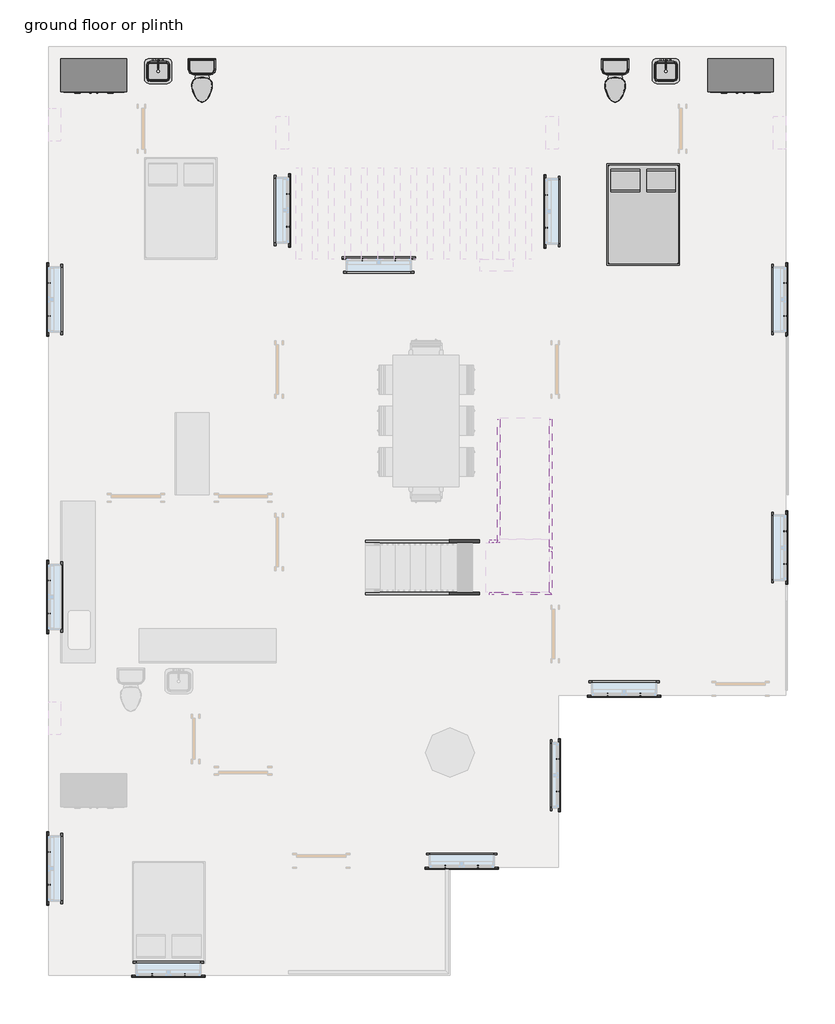
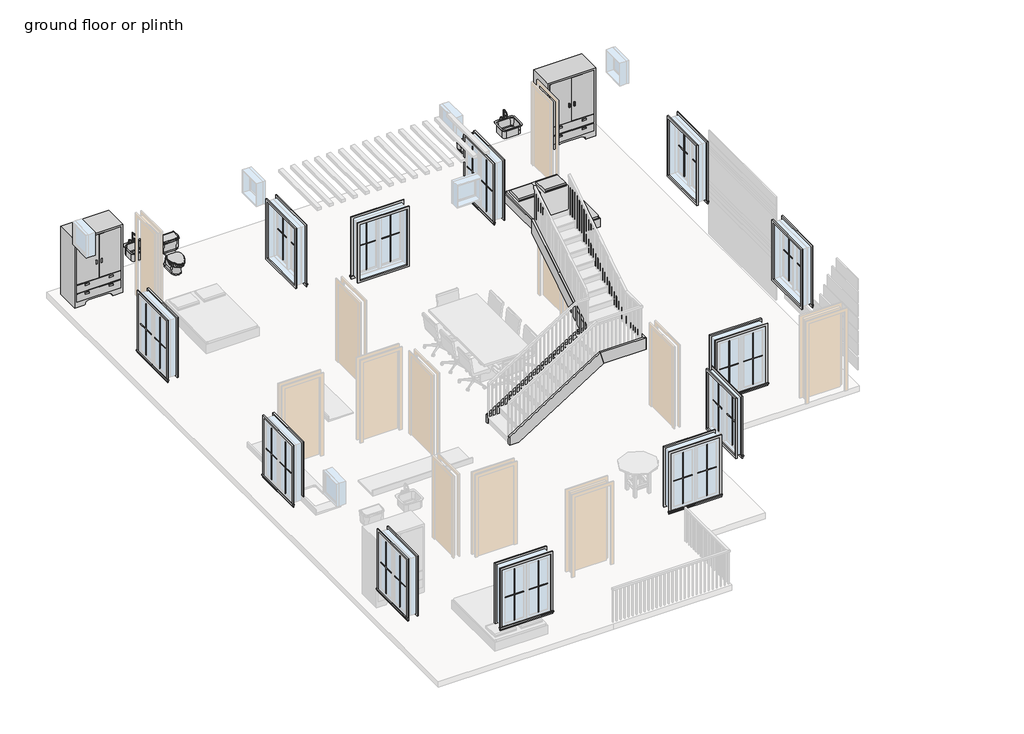
# One storey, part 3 of 3: 48 proxies, 7 members, 4 flow terminals, 3 furniture elements.
"""IFC4 building model written with IfcOpenShell, lengths in millimetres."""

from ifc_helpers import new_model, si_unit, frame, origin, place, context, project, spatial, polyline, outline, extrude, faceted_brep, transform, mapped, element, save
from components import muntin_pattern_2x2_muntin_pattern_2x2_6dad3731, muntin_pattern_2x2_muntin_pattern_2x2_a30a3345, trim_window_exterior_flat_with_sill_92b9b949, trim_window_interior_flat_picture_frame_3bb882cf, flow_terminal_8d9ea526, toilet_domestic_3d_toilet_domestic_3d_ba6479b0, toilet_domestic_3d_toilet_domestic_3d_30431060, furniture_b58f7881, furniture_82e269c4

model = new_model("IFC4")

# Units and contexts
model_context = context("Model", 3, world=origin())
ifc_project = project(units=[si_unit("LENGTHUNIT", "METRE", prefix="MILLI")], contexts=[model_context])

# Site, building, storey
site = spatial("IfcSite", under=ifc_project)
building = spatial("IfcBuilding", under=site)
storey = spatial("IfcBuildingStorey", under=building, Name="ground floor or plinth", Elevation=609.6)

# Proxies
placement = place(None, origin())
muntin_pattern_2x2_muntin_pattern_2x2_shape = muntin_pattern_2x2_muntin_pattern_2x2_6dad3731(model_context)
element("IfcBuildingElementProxy", 1, Name="Muntin Pattern_2x2 : Muntin Pattern_2x2", ObjectType="Muntin Pattern_2x2 : Muntin Pattern_2x2", at=placement, inside=storey, context=model_context, shape_type="MappedRepresentation", body=[
    mapped(muntin_pattern_2x2_muntin_pattern_2x2_shape, transform((3234.9048267, -163.1253076, 1593.85), x_axis=(-1.0, 0.0, 0.0), y_axis=(0.0, -1.0, 0.0), z_axis=(0.0, 0.0, 1.0))),
])
element("IfcBuildingElementProxy", 2, Name="Muntin Pattern_2x2 : Muntin Pattern_2x2", ObjectType="Muntin Pattern_2x2 : Muntin Pattern_2x2", at=placement, inside=storey, context=model_context, shape_type="MappedRepresentation", body=[
    mapped(muntin_pattern_2x2_muntin_pattern_2x2_shape, transform((718.7173267, 6534.5371924, 1593.85), x_axis=(0.0, 1.0, 0.0), y_axis=(-1.0, 0.0, 0.0), z_axis=(0.0, 0.0, 1.0))),
])
element("IfcBuildingElementProxy", 3, Name="Muntin Pattern_2x2 : Muntin Pattern_2x2", ObjectType="Muntin Pattern_2x2 : Muntin Pattern_2x2", at=placement, inside=storey, context=model_context, shape_type="MappedRepresentation", body=[
    mapped(muntin_pattern_2x2_muntin_pattern_2x2_shape, transform((718.7173267, 12046.3371924, 1593.85), x_axis=(0.0, 1.0, 0.0), y_axis=(-1.0, 0.0, 0.0), z_axis=(0.0, 0.0, 1.0))),
])
element("IfcBuildingElementProxy", 4, Name="Muntin Pattern_2x2 : Muntin Pattern_2x2", ObjectType="Muntin Pattern_2x2 : Muntin Pattern_2x2", at=placement, inside=storey, context=model_context, shape_type="MappedRepresentation", body=[
    mapped(muntin_pattern_2x2_muntin_pattern_2x2_shape, transform((5144.6673267, 14303.7621924, 1593.85), x_axis=(0.0, -1.0, 0.0), y_axis=(1.0, 0.0, 0.0), z_axis=(0.0, 0.0, 1.0))),
])
element("IfcBuildingElementProxy", 5, Name="Muntin Pattern_2x2 : Muntin Pattern_2x2", ObjectType="Muntin Pattern_2x2 : Muntin Pattern_2x2", at=placement, inside=storey, context=model_context, shape_type="MappedRepresentation", body=[
    mapped(muntin_pattern_2x2_muntin_pattern_2x2_shape, transform((9938.9173267, 13678.2871924, 1593.85), x_axis=(0.0, 1.0, 0.0), y_axis=(-1.0, 0.0, 0.0), z_axis=(0.0, 0.0, 1.0))),
])
element("IfcBuildingElementProxy", 6, Name="Muntin Pattern_2x2 : Muntin Pattern_2x2", ObjectType="Muntin Pattern_2x2 : Muntin Pattern_2x2", at=placement, inside=storey, context=model_context, shape_type="MappedRepresentation", body=[
    mapped(muntin_pattern_2x2_muntin_pattern_2x2_shape, transform((14364.8673267, 12652.7621924, 1593.85), x_axis=(0.0, -1.0, 0.0), y_axis=(1.0, 0.0, 0.0), z_axis=(0.0, 0.0, 1.0))),
])
element("IfcBuildingElementProxy", 7, Name="Muntin Pattern_2x2 : Muntin Pattern_2x2", ObjectType="Muntin Pattern_2x2 : Muntin Pattern_2x2", at=placement, inside=storey, context=model_context, shape_type="MappedRepresentation", body=[
    mapped(muntin_pattern_2x2_muntin_pattern_2x2_shape, transform((14364.8673267, 8055.3621924, 1593.85), x_axis=(0.0, -1.0, 0.0), y_axis=(1.0, 0.0, 0.0), z_axis=(0.0, 0.0, 1.0))),
])
element("IfcBuildingElementProxy", 8, Name="Muntin Pattern_2x2 : Muntin Pattern_2x2", ObjectType="Muntin Pattern_2x2 : Muntin Pattern_2x2", at=placement, inside=storey, context=model_context, shape_type="MappedRepresentation", body=[
    mapped(muntin_pattern_2x2_muntin_pattern_2x2_shape, transform((8670.5048267, 1843.4746924, 1593.85), x_axis=(-1.0, 0.0, 0.0), y_axis=(0.0, -1.0, 0.0), z_axis=(0.0, 0.0, 1.0))),
])
element("IfcBuildingElementProxy", 9, Name="Muntin Pattern_2x2 : Muntin Pattern_2x2", ObjectType="Muntin Pattern_2x2 : Muntin Pattern_2x2", at=placement, inside=storey, context=model_context, shape_type="MappedRepresentation", body=[
    mapped(muntin_pattern_2x2_muntin_pattern_2x2_shape, transform((10148.4673267, 3838.9621924, 1593.85), x_axis=(0.0, -1.0, 0.0), y_axis=(1.0, 0.0, 0.0), z_axis=(0.0, 0.0, 1.0))),
])
element("IfcBuildingElementProxy", 10, Name="Muntin Pattern_2x2 : Muntin Pattern_2x2", ObjectType="Muntin Pattern_2x2 : Muntin Pattern_2x2", at=placement, inside=storey, context=model_context, shape_type="MappedRepresentation", body=[
    mapped(muntin_pattern_2x2_muntin_pattern_2x2_shape, transform((6527.3798267, 13089.3246924, 1593.85), x_axis=(1.0, 0.0, 0.0), y_axis=(0.0, 1.0, 0.0), z_axis=(0.0, 0.0, 1.0))),
])
element("IfcBuildingElementProxy", 11, Name="Muntin Pattern_2x2 : Muntin Pattern_2x2", ObjectType="Muntin Pattern_2x2 : Muntin Pattern_2x2", at=placement, inside=storey, context=model_context, shape_type="MappedRepresentation", body=[
    mapped(muntin_pattern_2x2_muntin_pattern_2x2_shape, transform((718.7173267, 1505.3371924, 1593.85), x_axis=(0.0, 1.0, 0.0), y_axis=(-1.0, 0.0, 0.0), z_axis=(0.0, 0.0, 1.0))),
])
element("IfcBuildingElementProxy", 12, Name="Muntin Pattern_2x2 : Muntin Pattern_2x2", ObjectType="Muntin Pattern_2x2 : Muntin Pattern_2x2", at=placement, inside=storey, context=model_context, shape_type="MappedRepresentation", body=[
    mapped(muntin_pattern_2x2_muntin_pattern_2x2_shape, transform((11680.4048267, 5031.1746924, 1593.85), x_axis=(-1.0, 0.0, 0.0), y_axis=(0.0, -1.0, 0.0), z_axis=(0.0, 0.0, 1.0))),
])
muntin_pattern_2x2_muntin_pattern_2x2_2_shape = muntin_pattern_2x2_muntin_pattern_2x2_a30a3345(model_context)
element("IfcBuildingElementProxy", 13, Name="Muntin Pattern_2x2 : Muntin Pattern_2x2", ObjectType="Muntin Pattern_2x2 : Muntin Pattern_2x2", at=placement, inside=storey, context=model_context, shape_type="MappedRepresentation", body=[
    mapped(muntin_pattern_2x2_muntin_pattern_2x2_2_shape, transform((2628.4798267, -163.1253076, 1593.85), x_axis=(1.0, 0.0, 0.0), y_axis=(0.0, 1.0, 0.0), z_axis=(0.0, 0.0, 1.0))),
])
element("IfcBuildingElementProxy", 14, Name="Muntin Pattern_2x2 : Muntin Pattern_2x2", ObjectType="Muntin Pattern_2x2 : Muntin Pattern_2x2", at=placement, inside=storey, context=model_context, shape_type="MappedRepresentation", body=[
    mapped(muntin_pattern_2x2_muntin_pattern_2x2_2_shape, transform((718.7173267, 7140.9621924, 1593.85), x_axis=(0.0, -1.0, 0.0), y_axis=(1.0, 0.0, 0.0), z_axis=(0.0, 0.0, 1.0))),
])
element("IfcBuildingElementProxy", 15, Name="Muntin Pattern_2x2 : Muntin Pattern_2x2", ObjectType="Muntin Pattern_2x2 : Muntin Pattern_2x2", at=placement, inside=storey, context=model_context, shape_type="MappedRepresentation", body=[
    mapped(muntin_pattern_2x2_muntin_pattern_2x2_2_shape, transform((718.7173267, 12652.7621924, 1593.85), x_axis=(0.0, -1.0, 0.0), y_axis=(1.0, 0.0, 0.0), z_axis=(0.0, 0.0, 1.0))),
])
element("IfcBuildingElementProxy", 16, Name="Muntin Pattern_2x2 : Muntin Pattern_2x2", ObjectType="Muntin Pattern_2x2 : Muntin Pattern_2x2", at=placement, inside=storey, context=model_context, shape_type="MappedRepresentation", body=[
    mapped(muntin_pattern_2x2_muntin_pattern_2x2_2_shape, transform((5144.6673267, 13697.3371924, 1593.85), x_axis=(0.0, 1.0, 0.0), y_axis=(-1.0, 0.0, 0.0), z_axis=(0.0, 0.0, 1.0))),
])
element("IfcBuildingElementProxy", 17, Name="Muntin Pattern_2x2 : Muntin Pattern_2x2", ObjectType="Muntin Pattern_2x2 : Muntin Pattern_2x2", at=placement, inside=storey, context=model_context, shape_type="MappedRepresentation", body=[
    mapped(muntin_pattern_2x2_muntin_pattern_2x2_2_shape, transform((9938.9173267, 14284.7121924, 1593.85), x_axis=(0.0, -1.0, 0.0), y_axis=(1.0, 0.0, 0.0), z_axis=(0.0, 0.0, 1.0))),
])
element("IfcBuildingElementProxy", 18, Name="Muntin Pattern_2x2 : Muntin Pattern_2x2", ObjectType="Muntin Pattern_2x2 : Muntin Pattern_2x2", at=placement, inside=storey, context=model_context, shape_type="MappedRepresentation", body=[
    mapped(muntin_pattern_2x2_muntin_pattern_2x2_2_shape, transform((14364.8673267, 12046.3371924, 1593.85), x_axis=(0.0, 1.0, 0.0), y_axis=(-1.0, 0.0, 0.0), z_axis=(0.0, 0.0, 1.0))),
])
element("IfcBuildingElementProxy", 19, Name="Muntin Pattern_2x2 : Muntin Pattern_2x2", ObjectType="Muntin Pattern_2x2 : Muntin Pattern_2x2", at=placement, inside=storey, context=model_context, shape_type="MappedRepresentation", body=[
    mapped(muntin_pattern_2x2_muntin_pattern_2x2_2_shape, transform((14364.8673267, 7448.9371924, 1593.85), x_axis=(0.0, 1.0, 0.0), y_axis=(-1.0, 0.0, 0.0), z_axis=(0.0, 0.0, 1.0))),
])
element("IfcBuildingElementProxy", 20, Name="Muntin Pattern_2x2 : Muntin Pattern_2x2", ObjectType="Muntin Pattern_2x2 : Muntin Pattern_2x2", at=placement, inside=storey, context=model_context, shape_type="MappedRepresentation", body=[
    mapped(muntin_pattern_2x2_muntin_pattern_2x2_2_shape, transform((8064.0798267, 1843.4746924, 1593.85), x_axis=(1.0, 0.0, 0.0), y_axis=(0.0, 1.0, 0.0), z_axis=(0.0, 0.0, 1.0))),
])
element("IfcBuildingElementProxy", 21, Name="Muntin Pattern_2x2 : Muntin Pattern_2x2", ObjectType="Muntin Pattern_2x2 : Muntin Pattern_2x2", at=placement, inside=storey, context=model_context, shape_type="MappedRepresentation", body=[
    mapped(muntin_pattern_2x2_muntin_pattern_2x2_2_shape, transform((10148.4673267, 3232.5371924, 1593.85), x_axis=(0.0, 1.0, 0.0), y_axis=(-1.0, 0.0, 0.0), z_axis=(0.0, 0.0, 1.0))),
])
element("IfcBuildingElementProxy", 22, Name="Muntin Pattern_2x2 : Muntin Pattern_2x2", ObjectType="Muntin Pattern_2x2 : Muntin Pattern_2x2", at=placement, inside=storey, context=model_context, shape_type="MappedRepresentation", body=[
    mapped(muntin_pattern_2x2_muntin_pattern_2x2_2_shape, transform((7133.8048267, 13089.3246924, 1593.85), x_axis=(-1.0, 0.0, 0.0), y_axis=(0.0, -1.0, 0.0), z_axis=(0.0, 0.0, 1.0))),
])
element("IfcBuildingElementProxy", 23, Name="Muntin Pattern_2x2 : Muntin Pattern_2x2", ObjectType="Muntin Pattern_2x2 : Muntin Pattern_2x2", at=placement, inside=storey, context=model_context, shape_type="MappedRepresentation", body=[
    mapped(muntin_pattern_2x2_muntin_pattern_2x2_2_shape, transform((718.7173267, 2111.7621924, 1593.85), x_axis=(0.0, -1.0, 0.0), y_axis=(1.0, 0.0, 0.0), z_axis=(0.0, 0.0, 1.0))),
])
element("IfcBuildingElementProxy", 24, Name="Muntin Pattern_2x2 : Muntin Pattern_2x2", ObjectType="Muntin Pattern_2x2 : Muntin Pattern_2x2", at=placement, inside=storey, context=model_context, shape_type="MappedRepresentation", body=[
    mapped(muntin_pattern_2x2_muntin_pattern_2x2_2_shape, transform((11073.9798267, 5031.1746924, 1593.85), x_axis=(1.0, 0.0, 0.0), y_axis=(0.0, 1.0, 0.0), z_axis=(0.0, 0.0, 1.0))),
])
trim_window_exterior_flat_with_sill_shape = trim_window_exterior_flat_with_sill_92b9b949(model_context)
element("IfcBuildingElementProxy", 25, Name="Trim-Window-Exterior-Flat : with Sill", ObjectType="Trim-Window-Exterior-Flat : with Sill", at=placement, inside=storey, context=model_context, shape_type="MappedRepresentation", body=[
    mapped(trim_window_exterior_flat_with_sill_shape, transform((2931.6923267, -172.6503076, 3048.0), x_axis=(1.0, 0.0, 0.0), y_axis=(0.0, 0.0, 1.0), z_axis=(0.0, -1.0, 0.0))),
])
element("IfcBuildingElementProxy", 26, Name="Trim-Window-Exterior-Flat : with Sill", ObjectType="Trim-Window-Exterior-Flat : with Sill", at=placement, inside=storey, context=model_context, shape_type="MappedRepresentation", body=[
    mapped(trim_window_exterior_flat_with_sill_shape, transform((709.1923267, 6837.7496924, 3048.0), x_axis=(0.0, -1.0, 0.0), y_axis=(0.0, 0.0, 1.0), z_axis=(-1.0, 0.0, 0.0))),
])
element("IfcBuildingElementProxy", 27, Name="Trim-Window-Exterior-Flat : with Sill", ObjectType="Trim-Window-Exterior-Flat : with Sill", at=placement, inside=storey, context=model_context, shape_type="MappedRepresentation", body=[
    mapped(trim_window_exterior_flat_with_sill_shape, transform((709.1923267, 12349.5496924, 3048.0), x_axis=(0.0, -1.0, 0.0), y_axis=(0.0, 0.0, 1.0), z_axis=(-1.0, 0.0, 0.0))),
])
element("IfcBuildingElementProxy", 28, Name="Trim-Window-Exterior-Flat : with Sill", ObjectType="Trim-Window-Exterior-Flat : with Sill", at=placement, inside=storey, context=model_context, shape_type="MappedRepresentation", body=[
    mapped(trim_window_exterior_flat_with_sill_shape, transform((5154.1923267, 14000.5496924, 3048.0), x_axis=(0.0, 1.0, 0.0), y_axis=(0.0, 0.0, 1.0), z_axis=(1.0, 0.0, 0.0))),
])
element("IfcBuildingElementProxy", 29, Name="Trim-Window-Exterior-Flat : with Sill", ObjectType="Trim-Window-Exterior-Flat : with Sill", at=placement, inside=storey, context=model_context, shape_type="MappedRepresentation", body=[
    mapped(trim_window_exterior_flat_with_sill_shape, transform((9929.3923267, 13981.4996924, 3048.0), x_axis=(0.0, -1.0, 0.0), y_axis=(0.0, 0.0, 1.0), z_axis=(-1.0, 0.0, 0.0))),
])
element("IfcBuildingElementProxy", 30, Name="Trim-Window-Exterior-Flat : with Sill", ObjectType="Trim-Window-Exterior-Flat : with Sill", at=placement, inside=storey, context=model_context, shape_type="MappedRepresentation", body=[
    mapped(trim_window_exterior_flat_with_sill_shape, transform((14374.3923267, 12349.5496924, 3048.0), x_axis=(0.0, 1.0, 0.0), y_axis=(0.0, 0.0, 1.0), z_axis=(1.0, 0.0, 0.0))),
])
element("IfcBuildingElementProxy", 31, Name="Trim-Window-Exterior-Flat : with Sill", ObjectType="Trim-Window-Exterior-Flat : with Sill", at=placement, inside=storey, context=model_context, shape_type="MappedRepresentation", body=[
    mapped(trim_window_exterior_flat_with_sill_shape, transform((14374.3923267, 7752.1496924, 3048.0), x_axis=(0.0, 1.0, 0.0), y_axis=(0.0, 0.0, 1.0), z_axis=(1.0, 0.0, 0.0))),
])
element("IfcBuildingElementProxy", 32, Name="Trim-Window-Exterior-Flat : with Sill", ObjectType="Trim-Window-Exterior-Flat : with Sill", at=placement, inside=storey, context=model_context, shape_type="MappedRepresentation", body=[
    mapped(trim_window_exterior_flat_with_sill_shape, transform((8367.2923267, 1833.9496924, 3048.0), x_axis=(1.0, 0.0, 0.0), y_axis=(0.0, 0.0, 1.0), z_axis=(0.0, -1.0, 0.0))),
])
element("IfcBuildingElementProxy", 33, Name="Trim-Window-Exterior-Flat : with Sill", ObjectType="Trim-Window-Exterior-Flat : with Sill", at=placement, inside=storey, context=model_context, shape_type="MappedRepresentation", body=[
    mapped(trim_window_exterior_flat_with_sill_shape, transform((10157.9923267, 3535.7496924, 3048.0), x_axis=(0.0, 1.0, 0.0), y_axis=(0.0, 0.0, 1.0), z_axis=(1.0, 0.0, 0.0))),
])
element("IfcBuildingElementProxy", 34, Name="Trim-Window-Exterior-Flat : with Sill", ObjectType="Trim-Window-Exterior-Flat : with Sill", at=placement, inside=storey, context=model_context, shape_type="MappedRepresentation", body=[
    mapped(trim_window_exterior_flat_with_sill_shape, transform((6830.5923267, 13098.8496924, 3048.0), x_axis=(-1.0, 0.0, 0.0), y_axis=(0.0, 0.0, 1.0), z_axis=(0.0, 1.0, 0.0))),
])
element("IfcBuildingElementProxy", 35, Name="Trim-Window-Exterior-Flat : with Sill", ObjectType="Trim-Window-Exterior-Flat : with Sill", at=placement, inside=storey, context=model_context, shape_type="MappedRepresentation", body=[
    mapped(trim_window_exterior_flat_with_sill_shape, transform((709.1923267, 1808.5496924, 3048.0), x_axis=(0.0, -1.0, 0.0), y_axis=(0.0, 0.0, 1.0), z_axis=(-1.0, 0.0, 0.0))),
])
element("IfcBuildingElementProxy", 36, Name="Trim-Window-Exterior-Flat : with Sill", ObjectType="Trim-Window-Exterior-Flat : with Sill", at=placement, inside=storey, context=model_context, shape_type="MappedRepresentation", body=[
    mapped(trim_window_exterior_flat_with_sill_shape, transform((11377.1923267, 5021.6496924, 3048.0), x_axis=(1.0, 0.0, 0.0), y_axis=(0.0, 0.0, 1.0), z_axis=(0.0, -1.0, 0.0))),
])
trim_window_interior_flat_picture_frame_shape = trim_window_interior_flat_picture_frame_3bb882cf(model_context)
element("IfcBuildingElementProxy", 37, Name="Trim-Window-Interior-Flat : Picture Frame", ObjectType="Trim-Window-Interior-Flat : Picture Frame", at=placement, inside=storey, context=model_context, shape_type="MappedRepresentation", body=[
    mapped(trim_window_interior_flat_picture_frame_shape, transform((2931.6923267, 55.9496924, 3048.0), x_axis=(-1.0, 0.0, 0.0), y_axis=(0.0, 0.0, 1.0), z_axis=(0.0, 1.0, 0.0))),
])
element("IfcBuildingElementProxy", 38, Name="Trim-Window-Interior-Flat : Picture Frame", ObjectType="Trim-Window-Interior-Flat : Picture Frame", at=placement, inside=storey, context=model_context, shape_type="MappedRepresentation", body=[
    mapped(trim_window_interior_flat_picture_frame_shape, transform((937.7923267, 6837.7496924, 3048.0), x_axis=(0.0, 1.0, 0.0), y_axis=(0.0, 0.0, 1.0), z_axis=(1.0, 0.0, 0.0))),
])
element("IfcBuildingElementProxy", 39, Name="Trim-Window-Interior-Flat : Picture Frame", ObjectType="Trim-Window-Interior-Flat : Picture Frame", at=placement, inside=storey, context=model_context, shape_type="MappedRepresentation", body=[
    mapped(trim_window_interior_flat_picture_frame_shape, transform((937.7923267, 12349.5496924, 3048.0), x_axis=(0.0, 1.0, 0.0), y_axis=(0.0, 0.0, 1.0), z_axis=(1.0, 0.0, 0.0))),
])
element("IfcBuildingElementProxy", 40, Name="Trim-Window-Interior-Flat : Picture Frame", ObjectType="Trim-Window-Interior-Flat : Picture Frame", at=placement, inside=storey, context=model_context, shape_type="MappedRepresentation", body=[
    mapped(trim_window_interior_flat_picture_frame_shape, transform((4925.5923267, 14000.5496924, 3048.0), x_axis=(0.0, -1.0, 0.0), y_axis=(0.0, 0.0, 1.0), z_axis=(-1.0, 0.0, 0.0))),
])
element("IfcBuildingElementProxy", 41, Name="Trim-Window-Interior-Flat : Picture Frame", ObjectType="Trim-Window-Interior-Flat : Picture Frame", at=placement, inside=storey, context=model_context, shape_type="MappedRepresentation", body=[
    mapped(trim_window_interior_flat_picture_frame_shape, transform((10157.9923267, 13981.4996924, 3048.0), x_axis=(0.0, 1.0, 0.0), y_axis=(0.0, 0.0, 1.0), z_axis=(1.0, 0.0, 0.0))),
])
element("IfcBuildingElementProxy", 42, Name="Trim-Window-Interior-Flat : Picture Frame", ObjectType="Trim-Window-Interior-Flat : Picture Frame", at=placement, inside=storey, context=model_context, shape_type="MappedRepresentation", body=[
    mapped(trim_window_interior_flat_picture_frame_shape, transform((14145.7923267, 12349.5496924, 3048.0), x_axis=(0.0, -1.0, 0.0), y_axis=(0.0, 0.0, 1.0), z_axis=(-1.0, 0.0, 0.0))),
])
element("IfcBuildingElementProxy", 43, Name="Trim-Window-Interior-Flat : Picture Frame", ObjectType="Trim-Window-Interior-Flat : Picture Frame", at=placement, inside=storey, context=model_context, shape_type="MappedRepresentation", body=[
    mapped(trim_window_interior_flat_picture_frame_shape, transform((14145.7923267, 7752.1496924, 3048.0), x_axis=(0.0, -1.0, 0.0), y_axis=(0.0, 0.0, 1.0), z_axis=(-1.0, 0.0, 0.0))),
])
element("IfcBuildingElementProxy", 44, Name="Trim-Window-Interior-Flat : Picture Frame", ObjectType="Trim-Window-Interior-Flat : Picture Frame", at=placement, inside=storey, context=model_context, shape_type="MappedRepresentation", body=[
    mapped(trim_window_interior_flat_picture_frame_shape, transform((8367.2923267, 2062.5496924, 3048.0), x_axis=(-1.0, 0.0, 0.0), y_axis=(0.0, 0.0, 1.0), z_axis=(0.0, 1.0, 0.0))),
])
element("IfcBuildingElementProxy", 45, Name="Trim-Window-Interior-Flat : Picture Frame", ObjectType="Trim-Window-Interior-Flat : Picture Frame", at=placement, inside=storey, context=model_context, shape_type="MappedRepresentation", body=[
    mapped(trim_window_interior_flat_picture_frame_shape, transform((10043.6923267, 3535.7496924, 3048.0), x_axis=(0.0, -1.0, 0.0), y_axis=(0.0, 0.0, 1.0), z_axis=(-1.0, 0.0, 0.0))),
])
element("IfcBuildingElementProxy", 46, Name="Trim-Window-Interior-Flat : Picture Frame", ObjectType="Trim-Window-Interior-Flat : Picture Frame", at=placement, inside=storey, context=model_context, shape_type="MappedRepresentation", body=[
    mapped(trim_window_interior_flat_picture_frame_shape, transform((6830.5923267, 12870.2496924, 3048.0), x_axis=(1.0, 0.0, 0.0), y_axis=(0.0, 0.0, 1.0), z_axis=(0.0, -1.0, 0.0))),
])
element("IfcBuildingElementProxy", 47, Name="Trim-Window-Interior-Flat : Picture Frame", ObjectType="Trim-Window-Interior-Flat : Picture Frame", at=placement, inside=storey, context=model_context, shape_type="MappedRepresentation", body=[
    mapped(trim_window_interior_flat_picture_frame_shape, transform((937.7923267, 1808.5496924, 3048.0), x_axis=(0.0, 1.0, 0.0), y_axis=(0.0, 0.0, 1.0), z_axis=(1.0, 0.0, 0.0))),
])
element("IfcBuildingElementProxy", 48, Name="Trim-Window-Interior-Flat : Picture Frame", ObjectType="Trim-Window-Interior-Flat : Picture Frame", at=placement, inside=storey, context=model_context, shape_type="MappedRepresentation", body=[
    mapped(trim_window_interior_flat_picture_frame_shape, transform((11377.1923267, 5250.2496924, 3048.0), x_axis=(-1.0, 0.0, 0.0), y_axis=(0.0, 0.0, 1.0), z_axis=(0.0, 1.0, 0.0))),
])

# Flow terminals
flow_terminal_shape = flow_terminal_8d9ea526(model_context)
element("IfcFlowTerminal", 49, ObjectType="Sink Vanity-Square : 20\" x 18\"", at=placement, inside=storey, context=model_context, shape_type="MappedRepresentation", body=[
    mapped(flow_terminal_shape, transform((2725.5030862, 16627.1042913, 609.6), x_axis=(1.0, 0.0, 0.0), y_axis=(0.0, 1.0, 0.0), z_axis=(0.0, 0.0, 1.0))),
])
element("IfcFlowTerminal", 50, ObjectType="Sink Vanity-Square : 20\" x 18\"", at=placement, inside=storey, context=model_context, shape_type="MappedRepresentation", body=[
    mapped(flow_terminal_shape, transform((12136.2030862, 16627.1042913, 609.6), x_axis=(1.0, 0.0, 0.0), y_axis=(0.0, 1.0, 0.0), z_axis=(0.0, 0.0, 1.0))),
])
toilet_domestic_3d_toilet_domestic_3d_shape = toilet_domestic_3d_toilet_domestic_3d_ba6479b0(model_context)
toilet_domestic_3d_toilet_domestic_3d_2_shape = toilet_domestic_3d_toilet_domestic_3d_30431060(model_context)
element("IfcFlowTerminal", 51, ObjectType="Toilet-Domestic-3D : Toilet-Domestic-3D", at=placement, inside=storey, context=model_context, shape_type="MappedRepresentation", body=[
    mapped(toilet_domestic_3d_toilet_domestic_3d_shape, transform((3553.9923267, 16312.5536651, 609.6), x_axis=(1.0, 0.0, 0.0), y_axis=(0.0, 1.0, 0.0), z_axis=(0.0, 0.0, 1.0))),
    mapped(toilet_domestic_3d_toilet_domestic_3d_2_shape, transform((3553.9923267, 16312.5536651, 609.6), x_axis=(1.0, 0.0, 0.0), y_axis=(0.0, 1.0, 0.0), z_axis=(0.0, 0.0, 1.0))),
])
element("IfcFlowTerminal", 52, ObjectType="Toilet-Domestic-3D : Toilet-Domestic-3D", at=placement, inside=storey, context=model_context, shape_type="MappedRepresentation", body=[
    mapped(toilet_domestic_3d_toilet_domestic_3d_shape, transform((11212.0923267, 16312.5536651, 609.6), x_axis=(1.0, 0.0, 0.0), y_axis=(0.0, 1.0, 0.0), z_axis=(0.0, 0.0, 1.0))),
    mapped(toilet_domestic_3d_toilet_domestic_3d_2_shape, transform((11212.0923267, 16312.5536651, 609.6), x_axis=(1.0, 0.0, 0.0), y_axis=(0.0, 1.0, 0.0), z_axis=(0.0, 0.0, 1.0))),
])

# Furniture
furniture_shape = furniture_b58f7881(model_context)
element("IfcFurniture", 53, ObjectType="Bed-Box : Double 53\" x 74\"", at=placement, inside=storey, context=model_context, shape_type="MappedRepresentation", body=[
    mapped(furniture_shape, transform((11393.6398677, 14158.7792006, 609.6), x_axis=(1.0, 0.0, 0.0), y_axis=(0.0, 1.0, 0.0), z_axis=(0.0, 0.0, 1.0))),
])
furniture_2_shape = furniture_82e269c4(model_context)
element("IfcFurniture", 54, ObjectType="Wardrobe : 48\" x 72\" x 24\"", at=placement, inside=storey, context=model_context, shape_type="MappedRepresentation", body=[
    mapped(furniture_2_shape, transform((1816.5855866, 17086.188502, 609.6), x_axis=(1.0, 0.0, 0.0), y_axis=(0.0, 1.0, 0.0), z_axis=(0.0, 0.0, 1.0))),
])
element("IfcFurniture", 55, ObjectType="Wardrobe : 48\" x 72\" x 24\"", at=placement, inside=storey, context=model_context, shape_type="MappedRepresentation", body=[
    mapped(furniture_2_shape, transform((13805.3855866, 17086.188502, 609.6), x_axis=(1.0, 0.0, 0.0), y_axis=(0.0, 1.0, 0.0), z_axis=(0.0, 0.0, 1.0))),
])

# Members
element("IfcMember", 56, ObjectType="Stringer - 2\" Width", at=placement, inside=storey, context=model_context, shape_type="SweptSolid", body=[
    extrude(outline(polyline([(824.6106437, 6584.2175025), (609.6, 6584.2175025), (609.6, 6814.0730319), (1981.2, 8969.4444605), (2286.0, 8880.686491), (824.6106437, 6584.2175025)])), frame((0.0, 7843.0147181, 0.0), z_axis=(0.0, 1.0, 0.0), x_axis=(0.0, 0.0, 1.0)), (0.0, 0.0, 1.0), 50.8),
])
element("IfcMember", 57, ObjectType="Stringer - 2\" Width", at=placement, inside=storey, context=model_context, shape_type="SweptSolid", body=[
    extrude(outline(polyline([(824.6106437, 6584.2175025), (609.6, 6584.2175025), (609.6, 6814.0730319), (1981.2, 8969.4444605), (2286.0, 8880.686491), (824.6106437, 6584.2175025)])), frame((0.0, 6877.8147181, 0.0), z_axis=(0.0, 1.0, 0.0), x_axis=(0.0, 0.0, 1.0)), (0.0, 0.0, 1.0), 50.8),
])
element("IfcMember", 58, ObjectType="Stringer - 2\" Width", at=placement, inside=storey, context=model_context, shape_type="SweptSolid", body=[
    extrude(outline(polyline([(7843.0147181, 2031.2010268), (7843.0147181, 2392.483371), (10129.0147181, 3847.2106437), (10129.0147181, 3485.9282995), (7843.0147181, 2031.2010268)])), frame((9027.6923267, 0.0, 0.0), z_axis=(1.0, 0.0, 0.0), x_axis=(0.0, 1.0, 0.0)), (0.0, 0.0, 1.0), 50.8),
])
element("IfcMember", 59, ObjectType="Stringer - 2\" Width", at=placement, inside=storey, context=model_context, shape_type="SweptSolid", body=[
    extrude(outline(polyline([(7764.441676, 1981.2), (7675.6837065, 2286.0), (10129.0147181, 3847.2106437), (10129.0147181, 3485.9282995), (7764.441676, 1981.2)])), frame((9992.8923267, 0.0, 0.0), z_axis=(1.0, 0.0, 0.0), x_axis=(0.0, 1.0, 0.0)), (0.0, 0.0, 1.0), 50.8),
])
element("IfcMember", 60, ObjectType="Stringer - 2\" Width", at=placement, inside=storey, context=model_context, shape_type="Brep", body=[
    faceted_brep([(8880.686491, 6928.6147181, 2286.0), (8880.686491, 6877.8147181, 2286.0), (10043.6923267, 6877.8147181, 2286.0), (9992.8923267, 6928.6147181, 2286.0), (8969.4444605, 6928.6147181, 1981.2), (9992.8923267, 6928.6147181, 1981.2), (8969.4444605, 6877.8147181, 1981.2), (10043.6923267, 6877.8147181, 1981.2)], [[[0, 1, 2, 3]], [[4, 0, 3, 5]], [[6, 4, 5, 7]], [[1, 6, 7, 2]], [[1, 0, 4, 6]], [[2, 7, 5, 3]]]),
])
element("IfcMember", 61, ObjectType="Stringer - 2\" Width", at=placement, inside=storey, context=model_context, shape_type="SweptSolid", body=[
    extrude(outline(polyline([(1981.2, 9027.6923267), (2286.0, 9027.6923267), (2286.0, 8880.686491), (1981.2, 8969.4444605), (1981.2, 9027.6923267)])), frame((0.0, 7843.0147181, 0.0), z_axis=(0.0, 1.0, 0.0), x_axis=(0.0, 0.0, 1.0)), (0.0, 0.0, 1.0), 50.8),
])
element("IfcMember", 62, ObjectType="Stringer - 2\" Width", at=placement, inside=storey, context=model_context, shape_type="Brep", body=[
    faceted_brep([(9992.8923267, 6928.6147181, 2286.0), (10043.6923267, 6877.8147181, 2286.0), (10043.6923267, 7675.6837065, 2286.0), (9992.8923267, 7675.6837065, 2286.0), (9992.8923267, 6928.6147181, 1981.2), (9992.8923267, 7764.441676, 1981.2), (10043.6923267, 6877.8147181, 1981.2), (10043.6923267, 7764.441676, 1981.2)], [[[0, 1, 2, 3]], [[4, 0, 3, 5]], [[6, 4, 5, 7]], [[1, 6, 7, 2]], [[1, 0, 4, 6]], [[2, 7, 5, 3]]]),
])

save(model, "model.ifc")

# Revit data of these elements
# Type "Muntin Pattern_2x2 : Muntin Pattern_2x2"
#   Width [instance default] = 4' - 0"
#   Thickness = 0' - 0 1/2"
#   Height [instance default] = 4' - 0"
#   Distance = 0' - 0 3/4"
#   Interior Material [instance default] = none
#   Exterior Material [instance default] = none
#   Default Elevation = 0
# Type "Trim-Window-Exterior-Flat : with Sill"
#   Trim Width = 0' - 2 1/4"
#   Trim Thickness_Picture Frame = 0' - 1 1/4"
#   Trim Thickness_with Sill = 0' - 0 3/4"
#   Sill Thickness = 0' - 1 1/4"
#   Opening Width [instance default] = 2' - 0"
#   Opening Height [instance default] = 3' - 0"
#   Default Elevation = 4' - 0"
#   Sill = yes
#   Picture Frame = no
#   Trim Material [instance default] = none
# Type "Trim-Window-Interior-Flat : Picture Frame"
#   Trim Thickness_Picture Frame = 0' - 1 1/4"
#   Trim Width = 0' - 2 1/4"
#   Trim Thickness_with Sill = 0' - 0 3/4"
#   Sill Thickness = 0' - 1 1/4"
#   Opening Width [instance default] = 2' - 0"
#   Opening Height [instance default] = 3' - 0"
#   Default Elevation = 4' - 0"
#   Sill = no
#   Picture Frame = yes
#   Trim Material [instance default] = none
# Type "Sink Vanity-Square : 20\" x 18\""
#   Assembly Code = "D2010400"
#   Counter Height = 2' - 7"
#   Depth = 1' - 6"
#   Width = 1' - 8"
#   Basin Material = Porcelain, Linen
#   Faucet Material = Steel, Polished
#   Default Elevation = 0
# Type "Toilet-Domestic-3D : Toilet-Domestic-3D"
#   Assembly Code = "D2010110"
#   Toilet - Bowl/Basin Material = Porcelain, Linen
#   Toilet - Seat Material = Laminate, Linen, Matte
#   Default Elevation = 0
# Type "Bed-Box : Double 53\" x 74\""
#   Assembly Code = "E2020200"
#   Length = 6' - 2"
#   Width = 4' - 5"
#   Frame Material = Birch
#   Mattress Material = Linen, White
#   Default Elevation = 0
# Type "Wardrobe : 48\" x 72\" x 24\""
#   Assembly Code = "E2020200"
#   Depth = 2' - 0"
#   Height = 6' - 0"
#   Width = 4' - 0"
#   Material = Wood - Mahogany
#   Default Elevation = 0
# Elements 1, 2, 3, 4, 5, 6, 7, 8, 9, 10, 11, 12, 13, 14, 15, 16, 17, 18, 19, 20, 21, 22, 23, 24 (IfcBuildingElementProxy, "Muntin Pattern_2x2 : Muntin Pattern_2x2")
#   Width = 1' - 6 5/8"
#   Height = 4' - 6 1/2"
#   Interior Material = Wood - Stained
#   Exterior Material = Clad - White
#   Phase Created = New Construction
#   Materials on its faces: "Clad - White", "Wood - Stained"
# Elements 25, 26, 27, 28, 29, 30, 31, 32, 33, 34, 35, 36 (IfcBuildingElementProxy, "Trim-Window-Exterior-Flat : with Sill")
#   Opening Width = 4' - 0"
#   Opening Height = 5' - 0"
#   Trim Material = Clad - White
#   Phase Created = New Construction
#   Materials on its faces: "Clad - White"
# Elements 37, 38, 39, 40, 41, 42, 43, 44, 45, 46, 47, 48 (IfcBuildingElementProxy, "Trim-Window-Interior-Flat : Picture Frame")
#   Opening Width = 4' - 0"
#   Opening Height = 5' - 0"
#   Trim Material = Wood - Stained
#   Phase Created = New Construction
#   Materials on its faces: "Wood - Stained"
# Element 49 (IfcFlowTerminal, "Sink Vanity-Square : 20\" x 18\"")
#   Mark = "1"
#   Phase Created = New Construction
#   Materials on its faces: "Porcelain, Linen", "Steel, Polished"
# Element 50 (IfcFlowTerminal, "Sink Vanity-Square : 20\" x 18\"")
#   Mark = "2"
#   Phase Created = New Construction
#   Materials on its faces: "Porcelain, Linen", "Steel, Polished"
# Element 51 (IfcFlowTerminal, "Toilet-Domestic-3D : Toilet-Domestic-3D")
#   Mark = "4"
#   Phase Created = New Construction
#   Materials on its faces: "Porcelain, Linen", "Laminate, Linen, Matte"
# Element 52 (IfcFlowTerminal, "Toilet-Domestic-3D : Toilet-Domestic-3D")
#   Mark = "5"
#   Phase Created = New Construction
#   Materials on its faces: "Porcelain, Linen", "Laminate, Linen, Matte"
# Element 53 (IfcFurniture, "Bed-Box : Double 53\" x 74\"")
#   Phase Created = New Construction
#   Materials on its faces: "Birch", "Linen, White"
# Elements 54, 55 (IfcFurniture, "Wardrobe : 48\" x 72\" x 24\"")
#   Phase Created = New Construction
#   Materials on its faces: "Wood - Mahogany"
# Elements 56, 57, 58, 59, 60, 61, 62 (IfcMember, "Stringer - 2\" Width")
#   Phase Created = New Construction
# Materials
#   "Porcelain, Linen": class "Ceramic", colour RGB 249 239 230, transparency 0, Description = "Porcelain, linen", Cost = 0
#   "Steel, Polished": class "Metal", colour RGB 57 57 57, transparency 0, Description = "Polished steel", Cost = 0
#   "Laminate, Linen, Matte": class "Plastic", colour RGB 249 239 230, transparency 0, Description = "Plastic Laminate - Linen, Matte", Cost = 0
#   "Birch": class "Wood", colour RGB 224 178 126, transparency 0, Description = "Betula Alleghaniensis", Cost = 0
#   "Linen, White": class "Textile", colour RGB 247 247 239, transparency 0, Description = "Linen, white", Cost = 0
#   "Wood - Mahogany": colour RGB 138 86 45, transparency 0
#   "Clad - White": class "Wood", colour RGB 242 242 238, transparency 0, Cost = 0
#   "Wood - Stained": class "Wood", colour RGB 224 178 126, transparency 0, Cost = 0
